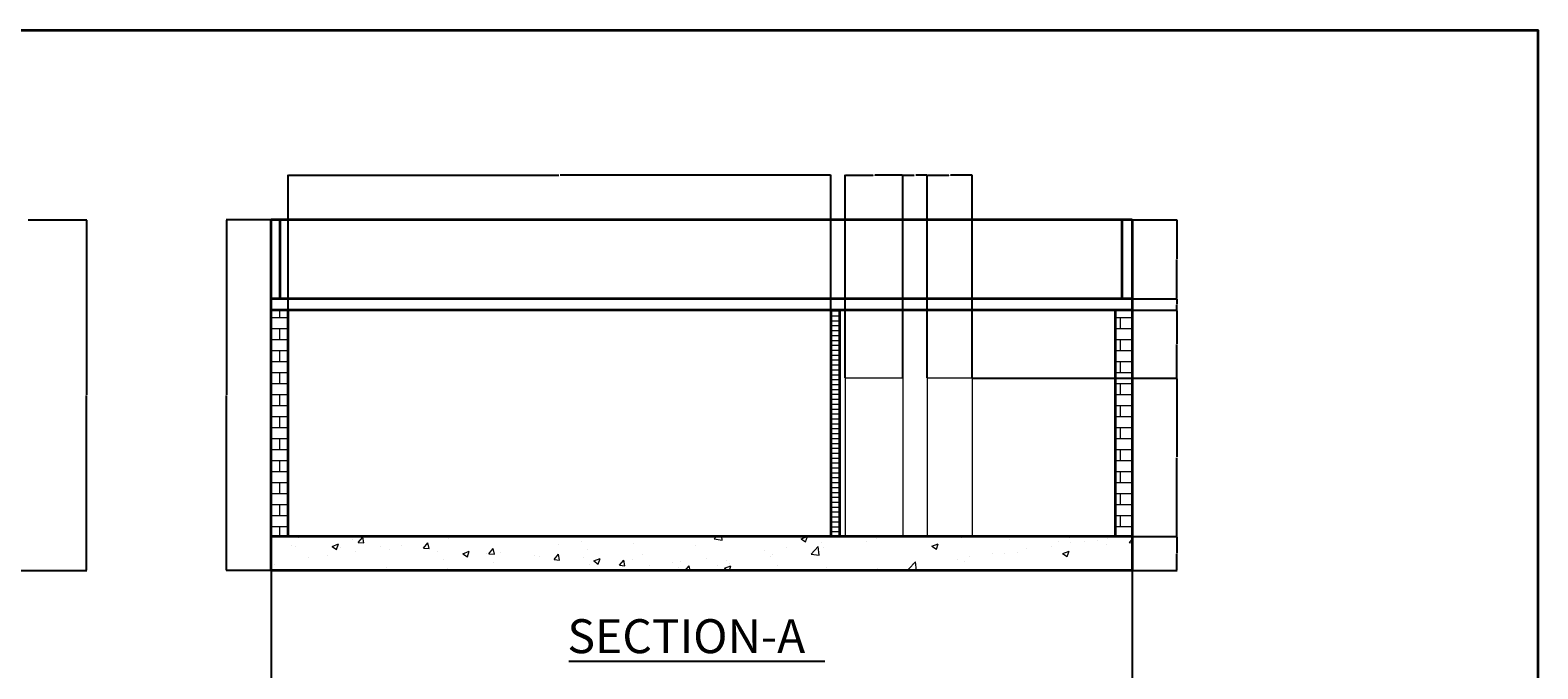
# Model space of a CAD drawing. Units: inches. Extents: x 2296 to 3812, y -1531 to 2564.
# Tile 10 of 10: x 3013 to 3812, y 2226 to 2564. Entities that reach past the tile are written whole.
import ezdxf

# ---------------------------------------------------------------- set-up
doc = ezdxf.new("R2010")
doc.units = ezdxf.units.IN
for name, color, linetype, lineweight in [('A-ANNO-DIMS', 2, 'Continuous', 18), ('A-ANNO-TEXT', 7, 'Continuous', 25), ('A-ANNO-TTLB', 7, 'Continuous', 35), ('A-FLOR-PATT', 252, 'Continuous', 13), ('A-SECT', 7, 'Continuous', 35), ('A-SECT-OPEN', 7, 'Continuous', 18), ('A-WALL-PATT', 252, 'Continuous', 13)]:
    doc.layers.add(name, color=color, linetype=linetype, lineweight=lineweight)
doc.styles.get("Standard").update_dxf_attribs({"font": 'arial.ttf'})
doc.dimstyles.get("Standard").update_dxf_attribs({"dimtxt": 0.18, "dimasz": 0.18, "dimexe": 0.18, "dimexo": 0.0625, "dimgap": 0.09, "dimtad": 0, "dimtih": 1, "dimtoh": 1, "dimdec": 4, "dimzin": 0, "dimdsep": 46, "dimtxsty": 'Standard', "dimcen": 0.09, "dimadec": 0, "dimazin": 0, "dimtfac": 1, "dimtdec": 4, "dimtofl": 0, "dimtmove": 0, "dimatfit": 3, "dimfxl": 1, "dimtolj": 1, "dimtzin": 0, "dimarcsym": 0})

# ---------------------------------------------------------------- blocks, each defined once
blk = doc.blocks.new('*D148')
at = {"layer": 'A-ANNO-DIMS', "color": 0, "lineweight": -2, "transparency": 16777216}
for p, q in [((3012.01, 2463.78), (3043.23, 2463.78)), ((3043.05, 2463.6), (3043.05, 2370.97)), ((3043.05, 2277.96), (3043.05, 2370.6)), ((2988.01, 2277.78), (3043.23, 2277.78))]:
    blk.add_line(p, q, dxfattribs=at)
at = {"layer": 'A-ANNO-DIMS', "color": 0, "transparency": 16777216}
for points in [[(3043.02, 2463.6), (3043.08, 2463.6), (3043.05, 2463.78)], [(3043.02, 2277.96), (3043.08, 2277.96), (3043.05, 2277.78)]]:
    blk.add_solid(points, dxfattribs=at)
at = {"layer": 'Defpoints', "color": 0, "transparency": 16777216}
for p in [(3011.95, 2463.78), (2987.95, 2277.78), (3043.05, 2277.78)]:
    blk.add_point(p, dxfattribs=at)
at = {"layer": 'A-ANNO-DIMS', "color": 0, "transparency": 16777216, "insert": (3043.05, 2370.78), "char_height": 0.18, "attachment_point": 5}
blk.add_mtext('\\A1;186', dxfattribs=at)
blk = doc.blocks.new('*D159')
at = {"layer": 'A-ANNO-DIMS', "color": 0, "lineweight": -2, "transparency": 16777216}
for p, q in [((3140.84, 2277.72), (3140.84, 2205.81)), ((3597.32, 2277.72), (3597.32, 2205.81)), ((3141.02, 2205.99), (3368.68, 2205.99)), ((3597.14, 2205.99), (3369.48, 2205.99))]:
    blk.add_line(p, q, dxfattribs=at)
at = {"layer": 'A-ANNO-DIMS', "color": 0, "transparency": 16777216}
for points in [[(3141.02, 2206.02), (3141.02, 2205.96), (3140.84, 2205.99)], [(3597.14, 2206.02), (3597.14, 2205.96), (3597.32, 2205.99)]]:
    blk.add_solid(points, dxfattribs=at)
at = {"layer": 'Defpoints', "color": 0, "transparency": 16777216}
for p in [(3140.84, 2277.78), (3597.32, 2277.78), (3597.32, 2205.99)]:
    blk.add_point(p, dxfattribs=at)
at = {"layer": 'A-ANNO-DIMS', "color": 0, "transparency": 16777216, "insert": (3369.08, 2205.99), "char_height": 0.18, "attachment_point": 5}
blk.add_mtext('\\A1;456.5', dxfattribs=at)
blk = doc.blocks.new('*D160')
at = {"layer": 'A-ANNO-DIMS', "color": 0, "lineweight": -2, "transparency": 16777216}
for p, q in [((3140.78, 2463.78), (3116.96, 2463.78)), ((3117.14, 2463.6), (3117.14, 2370.97)), ((3117.14, 2277.96), (3117.14, 2370.6)), ((3140.78, 2277.78), (3116.96, 2277.78))]:
    blk.add_line(p, q, dxfattribs=at)
at = {"layer": 'A-ANNO-DIMS', "color": 0, "transparency": 16777216}
for points in [[(3117.11, 2463.6), (3117.17, 2463.6), (3117.14, 2463.78)], [(3117.11, 2277.96), (3117.17, 2277.96), (3117.14, 2277.78)]]:
    blk.add_solid(points, dxfattribs=at)
at = {"layer": 'Defpoints', "color": 0, "transparency": 16777216}
for p in [(3117.14, 2463.78), (3140.84, 2463.78), (3140.84, 2277.78)]:
    blk.add_point(p, dxfattribs=at)
at = {"layer": 'A-ANNO-DIMS', "color": 0, "transparency": 16777216, "insert": (3117.14, 2370.78), "char_height": 0.18, "attachment_point": 5}
blk.add_mtext('\\A1;186', dxfattribs=at)
blk = doc.blocks.new('*D161')
at = {"layer": 'A-ANNO-DIMS', "color": 0, "lineweight": -2, "transparency": 16777216}
for p, q in [((3597.38, 2295.78), (3621.2, 2295.78)), ((3621.02, 2295.6), (3621.02, 2286.97)), ((3621.02, 2277.96), (3621.02, 2286.6)), ((3597.38, 2277.78), (3621.2, 2277.78))]:
    blk.add_line(p, q, dxfattribs=at)
at = {"layer": 'A-ANNO-DIMS', "color": 0, "transparency": 16777216}
for points in [[(3620.99, 2295.6), (3621.05, 2295.6), (3621.02, 2295.78)], [(3620.99, 2277.96), (3621.05, 2277.96), (3621.02, 2277.78)]]:
    blk.add_solid(points, dxfattribs=at)
at = {"layer": 'Defpoints', "color": 0, "transparency": 16777216}
for p in [(3597.32, 2295.78), (3621.02, 2295.78), (3597.32, 2277.78)]:
    blk.add_point(p, dxfattribs=at)
at = {"layer": 'A-ANNO-DIMS', "color": 0, "transparency": 16777216, "insert": (3621.02, 2286.78), "char_height": 0.18, "attachment_point": 5}
blk.add_mtext('\\A1;18', dxfattribs=at)
blk = doc.blocks.new('*D162')
at = {"layer": 'A-ANNO-DIMS', "color": 0, "lineweight": -2, "transparency": 16777216}
for p, q in [((3149.84, 2415.85), (3149.84, 2487.66)), ((3150.02, 2487.48), (3293.35, 2487.48)), ((3437.48, 2487.48), (3294.15, 2487.48)), ((3437.66, 2415.85), (3437.66, 2487.66))]:
    blk.add_line(p, q, dxfattribs=at)
at = {"layer": 'A-ANNO-DIMS', "color": 0, "transparency": 16777216}
for points in [[(3150.02, 2487.51), (3150.02, 2487.45), (3149.84, 2487.48)], [(3437.48, 2487.51), (3437.48, 2487.45), (3437.66, 2487.48)]]:
    blk.add_solid(points, dxfattribs=at)
at = {"layer": 'Defpoints', "color": 0, "transparency": 16777216}
for p in [(3437.66, 2487.48), (3149.84, 2415.78), (3437.66, 2415.78)]:
    blk.add_point(p, dxfattribs=at)
at = {"layer": 'A-ANNO-DIMS', "color": 0, "transparency": 16777216, "insert": (3293.75, 2487.48), "char_height": 0.18, "attachment_point": 5}
blk.add_mtext('\\A1;287.8', dxfattribs=at)
blk = doc.blocks.new('*D163')
at = {"layer": 'A-ANNO-DIMS', "color": 0, "lineweight": -2, "transparency": 16777216}
for p, q in [((3597.38, 2463.78), (3621.2, 2463.78)), ((3621.02, 2463.6), (3621.02, 2442.97)), ((3621.02, 2421.96), (3621.02, 2442.6)), ((3597.38, 2421.78), (3621.2, 2421.78))]:
    blk.add_line(p, q, dxfattribs=at)
at = {"layer": 'A-ANNO-DIMS', "color": 0, "transparency": 16777216}
for points in [[(3620.99, 2463.6), (3621.05, 2463.6), (3621.02, 2463.78)], [(3620.99, 2421.96), (3621.05, 2421.96), (3621.02, 2421.78)]]:
    blk.add_solid(points, dxfattribs=at)
at = {"layer": 'Defpoints', "color": 0, "transparency": 16777216}
for p in [(3597.32, 2463.78), (3621.02, 2463.78), (3597.32, 2421.78)]:
    blk.add_point(p, dxfattribs=at)
at = {"layer": 'A-ANNO-DIMS', "color": 0, "transparency": 16777216, "insert": (3621.02, 2442.78), "char_height": 0.18, "attachment_point": 5}
blk.add_mtext('\\A1;42', dxfattribs=at)
blk = doc.blocks.new('*D164')
at = {"layer": 'A-ANNO-DIMS', "color": 0, "lineweight": -2, "transparency": 16777216}
for p, q in [((3597.38, 2421.78), (3621.2, 2421.78)), ((3597.38, 2415.78), (3621.2, 2415.78)), ((3621.02, 2421.6), (3621.02, 2418.97)), ((3621.02, 2415.96), (3621.02, 2418.6))]:
    blk.add_line(p, q, dxfattribs=at)
at = {"layer": 'A-ANNO-DIMS', "color": 0, "transparency": 16777216}
for points in [[(3620.99, 2421.6), (3621.05, 2421.6), (3621.02, 2421.78)], [(3620.99, 2415.96), (3621.05, 2415.96), (3621.02, 2415.78)]]:
    blk.add_solid(points, dxfattribs=at)
at = {"layer": 'Defpoints', "color": 0, "transparency": 16777216}
for p in [(3597.32, 2421.78), (3597.32, 2415.78), (3621.02, 2421.78)]:
    blk.add_point(p, dxfattribs=at)
at = {"layer": 'A-ANNO-DIMS', "color": 0, "transparency": 16777216, "insert": (3621.02, 2418.78), "char_height": 0.18, "attachment_point": 5}
blk.add_mtext('\\A1;6', dxfattribs=at)
blk = doc.blocks.new('*D165')
at = {"layer": 'A-ANNO-DIMS', "color": 0, "lineweight": -2, "transparency": 16777216}
for p, q in [((3512.65, 2379.78), (3621.2, 2379.78)), ((3621.02, 2379.6), (3621.02, 2337.97)), ((3621.02, 2295.96), (3621.02, 2337.6)), ((3512.65, 2295.78), (3621.2, 2295.78))]:
    blk.add_line(p, q, dxfattribs=at)
at = {"layer": 'A-ANNO-DIMS', "color": 0, "transparency": 16777216}
for points in [[(3620.99, 2379.6), (3621.05, 2379.6), (3621.02, 2379.78)], [(3620.99, 2295.96), (3621.05, 2295.96), (3621.02, 2295.78)]]:
    blk.add_solid(points, dxfattribs=at)
at = {"layer": 'Defpoints', "color": 0, "transparency": 16777216}
for p in [(3512.59, 2379.78), (3512.59, 2295.78), (3621.02, 2295.78)]:
    blk.add_point(p, dxfattribs=at)
at = {"layer": 'A-ANNO-DIMS', "color": 0, "transparency": 16777216, "insert": (3621.02, 2337.78), "char_height": 0.18, "attachment_point": 5}
blk.add_mtext('\\A1;84', dxfattribs=at)
blk = doc.blocks.new('*D166')
at = {"layer": 'A-ANNO-DIMS', "color": 0, "lineweight": -2, "transparency": 16777216}
for p, q in [((3597.38, 2415.78), (3621.2, 2415.78)), ((3621.02, 2415.6), (3621.02, 2397.97)), ((3621.02, 2379.96), (3621.02, 2397.6)), ((3512.65, 2379.78), (3621.2, 2379.78))]:
    blk.add_line(p, q, dxfattribs=at)
at = {"layer": 'A-ANNO-DIMS', "color": 0, "transparency": 16777216}
for points in [[(3620.99, 2415.6), (3621.05, 2415.6), (3621.02, 2415.78)], [(3620.99, 2379.96), (3621.05, 2379.96), (3621.02, 2379.78)]]:
    blk.add_solid(points, dxfattribs=at)
at = {"layer": 'Defpoints', "color": 0, "transparency": 16777216}
for p in [(3597.32, 2415.78), (3621.02, 2415.78), (3512.59, 2379.78)]:
    blk.add_point(p, dxfattribs=at)
at = {"layer": 'A-ANNO-DIMS', "color": 0, "transparency": 16777216, "insert": (3621.02, 2397.78), "char_height": 0.18, "attachment_point": 5}
blk.add_mtext('\\A1;36', dxfattribs=at)
blk = doc.blocks.new('*D167')
at = {"layer": 'A-ANNO-DIMS', "color": 0, "lineweight": -2, "transparency": 16777216}
for p, q in [((3445.21, 2379.85), (3445.21, 2487.66)), ((3445.39, 2487.48), (3460.09, 2487.48)), ((3475.59, 2487.48), (3460.88, 2487.48)), ((3475.77, 2379.85), (3475.77, 2487.66))]:
    blk.add_line(p, q, dxfattribs=at)
at = {"layer": 'A-ANNO-DIMS', "color": 0, "transparency": 16777216}
for points in [[(3445.39, 2487.51), (3445.39, 2487.45), (3445.21, 2487.48)], [(3475.59, 2487.51), (3475.59, 2487.45), (3475.77, 2487.48)]]:
    blk.add_solid(points, dxfattribs=at)
at = {"layer": 'Defpoints', "color": 0, "transparency": 16777216}
for p in [(3475.77, 2487.48), (3445.21, 2379.78), (3475.77, 2379.78)]:
    blk.add_point(p, dxfattribs=at)
at = {"layer": 'A-ANNO-DIMS', "color": 0, "transparency": 16777216, "insert": (3460.49, 2487.48), "char_height": 0.18, "attachment_point": 5}
blk.add_mtext('\\A1;30.56', dxfattribs=at)
blk = doc.blocks.new('*D168')
at = {"layer": 'A-ANNO-DIMS', "color": 0, "lineweight": -2, "transparency": 16777216}
for p, q in [((3488.7, 2379.85), (3488.7, 2487.66)), ((3488.88, 2487.48), (3500.18, 2487.48)), ((3512.41, 2487.48), (3501.11, 2487.48)), ((3512.59, 2379.85), (3512.59, 2487.66))]:
    blk.add_line(p, q, dxfattribs=at)
at = {"layer": 'A-ANNO-DIMS', "color": 0, "transparency": 16777216}
for points in [[(3488.88, 2487.51), (3488.88, 2487.45), (3488.7, 2487.48)], [(3512.41, 2487.51), (3512.41, 2487.45), (3512.59, 2487.48)]]:
    blk.add_solid(points, dxfattribs=at)
at = {"layer": 'Defpoints', "color": 0, "transparency": 16777216}
for p in [(3512.59, 2487.48), (3488.7, 2379.78), (3512.59, 2379.78)]:
    blk.add_point(p, dxfattribs=at)
at = {"layer": 'A-ANNO-DIMS', "color": 0, "transparency": 16777216, "insert": (3500.65, 2487.48), "char_height": 0.18, "attachment_point": 5}
blk.add_mtext('\\A1;23.886', dxfattribs=at)
blk = doc.blocks.new('*D169')
at = {"layer": 'A-ANNO-DIMS', "color": 0, "lineweight": -2, "transparency": 16777216}
for p, q in [((3475.77, 2379.85), (3475.77, 2487.66)), ((3475.95, 2487.48), (3481.78, 2487.48)), ((3488.52, 2487.48), (3482.69, 2487.48)), ((3488.7, 2379.85), (3488.7, 2487.66))]:
    blk.add_line(p, q, dxfattribs=at)
at = {"layer": 'A-ANNO-DIMS', "color": 0, "transparency": 16777216}
for points in [[(3475.95, 2487.51), (3475.95, 2487.45), (3475.77, 2487.48)], [(3488.52, 2487.51), (3488.52, 2487.45), (3488.7, 2487.48)]]:
    blk.add_solid(points, dxfattribs=at)
at = {"layer": 'Defpoints', "color": 0, "transparency": 16777216}
for p in [(3488.7, 2487.48), (3475.77, 2379.78), (3488.7, 2379.78)]:
    blk.add_point(p, dxfattribs=at)
at = {"layer": 'A-ANNO-DIMS', "color": 0, "transparency": 16777216, "insert": (3482.24, 2487.48), "char_height": 0.18, "attachment_point": 5}
blk.add_mtext('\\A1;12.935', dxfattribs=at)

msp = doc.modelspace()

# ---------------------------------------------------------------- hatches: boundary and pattern name
at = {"layer": 'A-FLOR-PATT'}
h = msp.add_hatch(dxfattribs=at)
h.set_pattern_fill('AR-CONC', color=256, scale=0.19, style=0)
h.paths.add_polyline_path([(3140.8418, 2277.7848), (3597.3177, 2277.7848), (3597.3177, 2295.7848), (3140.8418, 2295.7848)])
at = {"layer": 'A-WALL-PATT'}
h = msp.add_hatch(dxfattribs=at)
h.set_pattern_fill('AR-BRSTD', color=256, scale=0.086, style=0)
h.paths.add_polyline_path([(3140.8418, 2295.7848), (3149.8418, 2295.7848), (3149.8418, 2415.7848), (3140.8418, 2415.7848)])
h = msp.add_hatch(dxfattribs=at)
h.set_pattern_fill('ANSI31', color=256, scale=0.818898, angle=-45, style=0)
h.paths.add_polyline_path([(3437.6588, 2295.7848), (3442.1588, 2295.7848), (3442.1588, 2415.7848), (3437.6588, 2415.7848)])
h = msp.add_hatch(dxfattribs=at)
h.set_pattern_fill('AR-BRSTD', color=256, scale=0.086, style=0)
h.paths.add_polyline_path([(3588.3177, 2295.7848), (3597.3177, 2295.7848), (3597.3177, 2415.7848), (3588.3177, 2415.7848)])

# ---------------------------------------------------------------- linework, layer by layer
at = {"layer": 'A-ANNO-TEXT'}
msp.add_line((3298.7865, 2229.6928), (3434.3633, 2229.6928), dxfattribs=at)
at = {"layer": 'A-ANNO-TTLB'}
msp.add_lwpolyline([(2296.1257, 2564.2989), (3812.4193, 2564.2989), (3812.4193, 1124.0028), (2296.1257, 1124.0028)], close=True, dxfattribs=at)
at = {"layer": 'A-SECT'}
for p, q in [((3597.3177, 2463.7848), (3140.8418, 2463.7848)), ((3140.8418, 2277.7848), (3140.8418, 2463.7848)), ((3145.6041, 2421.7848), (3145.6041, 2463.7848)), ((3592.0093, 2421.7848), (3592.0093, 2463.7848)), ((3597.3177, 2463.7848), (3597.3177, 2277.7848)), ((3597.3177, 2421.7848), (3140.8418, 2421.7848)), ((3597.3177, 2415.7848), (3140.8418, 2415.7848)), ((3149.8418, 2295.7848), (3149.8418, 2415.7848)), ((3437.6588, 2415.7848), (3437.6588, 2295.7848)), ((3442.1588, 2415.7848), (3442.1588, 2295.7848)), ((3588.3177, 2415.7848), (3588.3177, 2295.7848)), ((3597.3177, 2295.7848), (3140.8418, 2295.7848)), ((3597.3177, 2277.7848), (3140.8418, 2277.7848))]:
    msp.add_line(p, q, dxfattribs=at)
at = {"layer": 'A-SECT-OPEN'}
for p, q in [((3445.2067, 2379.7848), (3445.2067, 2295.7848)), ((3475.769, 2379.7848), (3445.2067, 2379.7848)), ((3475.769, 2379.7848), (3475.769, 2295.7848)), ((3488.7043, 2379.7848), (3488.7043, 2295.7848)), ((3512.59, 2379.7848), (3488.7043, 2379.7848)), ((3512.59, 2379.7848), (3512.59, 2295.7848))]:
    msp.add_line(p, q, dxfattribs=at)

# ---------------------------------------------------------------- texts
at = {"layer": 'A-ANNO-TEXT', "insert": (3297.9416, 2251.9458), "char_height": 18, "attachment_point": 1}
msp.add_mtext_dynamic_manual_height_columns('SECTION-A', width=284.863043, gutter_width=12.5, heights=[0], dxfattribs=at)

# ---------------------------------------------------------------- dimensions: what is measured, and where the dimension line sits
at = {"layer": 'A-ANNO-DIMS'}
for base, p1, p2, override, picture, middle in [((3437.6588, 2487.4848), (3149.8418, 2415.7848), (3437.6588, 2415.7848), {"dimdec": 1, "dimlfac": 1, "dimrnd": 0, "dimzin": 0, "dimdsep": 46, "dimlunit": 2}, '*D162', (3293.7503, 2487.4848)), ((3475.769, 2487.4848), (3445.2067, 2379.7848), (3475.769, 2379.7848), {"dimdec": 2, "dimlfac": 1, "dimrnd": 0, "dimzin": 0, "dimdsep": 46, "dimlunit": 2}, '*D167', (3460.4879, 2487.4848)), ((3488.7043, 2487.4848), (3475.769, 2379.7848), (3488.7043, 2379.7848), {"dimdec": 3, "dimlfac": 1, "dimrnd": 0, "dimzin": 0, "dimdsep": 46, "dimlunit": 2}, '*D169', (3482.2367, 2487.4848)), ((3512.59, 2487.4848), (3488.7043, 2379.7848), (3512.59, 2379.7848), {"dimdec": 3, "dimlfac": 1, "dimrnd": 0, "dimzin": 0, "dimdsep": 46, "dimlunit": 2}, '*D168', (3500.6471, 2487.4848)), ((3597.3177, 2205.9928), (3140.8418, 2277.7848), (3597.3177, 2277.7848), {"dimdec": 1, "dimlfac": 1, "dimrnd": 0, "dimzin": 0, "dimdsep": 46, "dimlunit": 2}, '*D159', (3369.0797, 2205.9928))]:
    dim = msp.add_linear_dim(base=base, p1=p1, p2=p2, dimstyle='Standard', override=override, dxfattribs=at)
    dim.commit()
    dim.dimension.update_dxf_attribs({"geometry": picture, "text_midpoint": middle})
for base, p1, p2, picture, middle in [((3043.0477, 2277.7848), (3011.9477, 2463.7848), (2987.9477, 2277.7848), '*D148', (3043.0477, 2370.7848)), ((3117.1418, 2463.7848), (3140.8418, 2277.7848), (3140.8418, 2463.7848), '*D160', (3117.1418, 2370.7848)), ((3621.0177, 2463.7848), (3597.3177, 2421.7848), (3597.3177, 2463.7848), '*D163', (3621.0177, 2442.7848)), ((3621.0177, 2415.7848), (3512.59, 2379.7848), (3597.3177, 2415.7848), '*D166', (3621.0177, 2397.7848)), ((3621.0177, 2421.7848), (3597.3177, 2415.7848), (3597.3177, 2421.7848), '*D164', (3621.0177, 2418.7848)), ((3621.0177, 2295.7848), (3512.59, 2379.7848), (3512.59, 2295.7848), '*D165', (3621.0177, 2337.7848)), ((3621.0177, 2295.7848), (3597.3177, 2277.7848), (3597.3177, 2295.7848), '*D161', (3621.0177, 2286.7848))]:
    dim = msp.add_linear_dim(base=base, p1=p1, p2=p2, angle=90, dimstyle='Standard', override={"dimdec": 0, "dimlfac": 1, "dimrnd": 0, "dimzin": 0, "dimdsep": 46, "dimlunit": 2}, dxfattribs=at)
    dim.commit()
    dim.dimension.update_dxf_attribs({"geometry": picture, "text_midpoint": middle})

doc.saveas('drawing.dxf')
